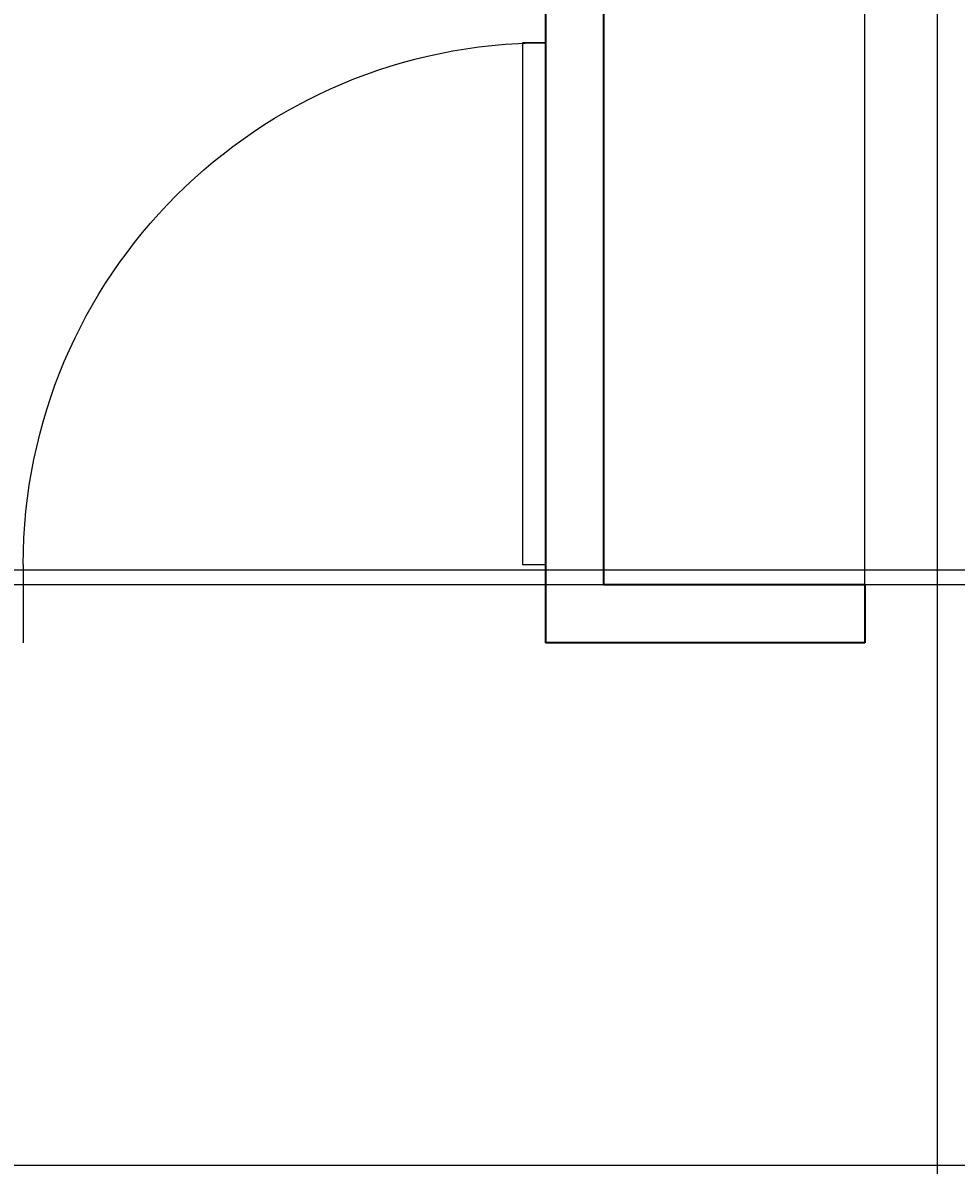
# Model space of a CAD drawing. Units: feet. Extents: x 105 to 1094, y -88 to 588.
# Tile 26 of 59: x 308 to 372, y 354 to 433. Entities that reach past the tile are written whole.
import ezdxf

# ---------------------------------------------------------------- set-up
doc = ezdxf.new("R2010")
doc.units = ezdxf.units.FT
doc.header["$MEASUREMENT"] = 0
for name, color, linetype, lineweight in [('A-ANNO-DIMS', 2, 'Continuous', 18), ('A-DOOR', 3, 'Continuous', 25), ('A-WALL', 7, 'Continuous', 35)]:
    doc.layers.add(name, color=color, linetype=linetype, lineweight=lineweight)
doc.styles.get("Standard").update_dxf_attribs({"font": 'arial.ttf'})
doc.dimstyles.get("Standard").update_dxf_attribs({"dimtxt": 0.18, "dimasz": 0.18, "dimexe": 0.18, "dimexo": 0.0625, "dimgap": 0.09, "dimtad": 0, "dimtih": 1, "dimtoh": 1, "dimdec": 4, "dimzin": 0, "dimdsep": 46, "dimtxsty": 'Standard', "dimcen": 0.09, "dimadec": 0, "dimazin": 0, "dimtfac": 1, "dimtdec": 4, "dimtofl": 0, "dimtmove": 0, "dimatfit": 3, "dimfxl": 1, "dimtolj": 1, "dimtzin": 0, "dimarcsym": 0})

# ---------------------------------------------------------------- blocks, each defined once
blk = doc.blocks.new('*U2')
for p, q in [((0, 0), (0, -6)), ((40, 0), (40, -6))]:
    blk.add_line(p, q)
blk.add_lwpolyline([(0, 0), (0, 40), (1.75, 40), (1.75, 0)], close=True)
blk.add_arc((0, 0), 40, 0, 90)
blk = doc.blocks.new('*D21')
at = {"layer": 'A-ANNO-DIMS', "color": 0, "lineweight": -2, "transparency": 16777216}
for p, q in [((849.626, 543.081), (105.458, 543.081)), ((105.638, 542.901), (105.638, 250.263)), ((105.638, -42.739), (105.638, 249.899)), ((849.626, -42.919), (105.458, -42.919))]:
    blk.add_line(p, q, dxfattribs=at)
at = {"layer": 'A-ANNO-DIMS', "color": 0, "transparency": 16777216}
for points in [[(105.608, 542.901), (105.668, 542.901), (105.638, 543.081)], [(105.608, -42.739), (105.668, -42.739), (105.638, -42.919)]]:
    blk.add_solid(points, dxfattribs=at)
at = {"layer": 'Defpoints', "color": 0, "transparency": 16777216}
for p in [(105.638, 543.081), (849.688, 543.081), (849.688, -42.919)]:
    blk.add_point(p, dxfattribs=at)
at = {"layer": 'A-ANNO-DIMS', "color": 0, "transparency": 16777216, "insert": (105.638, 250.081), "char_height": 0.18, "attachment_point": 5}
blk.add_mtext('\\A1;586', dxfattribs=at)
blk = doc.blocks.new('*D33')
at = {"layer": 'A-ANNO-DIMS', "color": 0, "lineweight": -2, "transparency": 16777216}
for p, q in [((646.626, 395.081), (105.458, 395.081)), ((105.638, 394.901), (105.638, 345.263)), ((105.638, 295.261), (105.638, 344.899)), ((646.626, 295.081), (105.458, 295.081))]:
    blk.add_line(p, q, dxfattribs=at)
at = {"layer": 'A-ANNO-DIMS', "color": 0, "transparency": 16777216}
for points in [[(105.608, 394.901), (105.668, 394.901), (105.638, 395.081)], [(105.608, 295.261), (105.668, 295.261), (105.638, 295.081)]]:
    blk.add_solid(points, dxfattribs=at)
at = {"layer": 'Defpoints', "color": 0, "transparency": 16777216}
for p in [(646.688, 395.081), (105.638, 295.081), (646.688, 295.081)]:
    blk.add_point(p, dxfattribs=at)
at = {"layer": 'A-ANNO-DIMS', "color": 0, "transparency": 16777216, "insert": (105.638, 345.081), "char_height": 0.18, "attachment_point": 5}
blk.add_mtext('\\A1;100', dxfattribs=at)
blk = doc.blocks.new('*D39')
at = {"layer": 'A-ANNO-DIMS', "color": 0, "lineweight": -2, "transparency": 16777216}
for p, q in [((294.688, 204.144), (294.688, 588.311)), ((294.868, 588.131), (332.47, 588.131)), ((370.508, 588.131), (332.906, 588.131)), ((370.688, 204.144), (370.688, 588.311))]:
    blk.add_line(p, q, dxfattribs=at)
at = {"layer": 'A-ANNO-DIMS', "color": 0, "transparency": 16777216}
for points in [[(294.868, 588.161), (294.868, 588.101), (294.688, 588.131)], [(370.508, 588.161), (370.508, 588.101), (370.688, 588.131)]]:
    blk.add_solid(points, dxfattribs=at)
at = {"layer": 'Defpoints', "color": 0, "transparency": 16777216}
for p in [(370.688, 588.131), (294.688, 204.081), (370.688, 204.081)]:
    blk.add_point(p, dxfattribs=at)
at = {"layer": 'A-ANNO-DIMS', "color": 0, "transparency": 16777216, "insert": (332.688, 588.131), "char_height": 0.18, "attachment_point": 5}
blk.add_mtext('\\A1;76', dxfattribs=at)
blk = doc.blocks.new('*D51')
at = {"layer": 'A-ANNO-DIMS', "color": 0, "lineweight": -2, "transparency": 16777216}
for p, q in [((432.626, 394.081), (105.458, 394.081)), ((105.638, 393.901), (105.638, 374.263)), ((105.638, 354.261), (105.638, 373.899)), ((426.626, 354.081), (105.458, 354.081))]:
    blk.add_line(p, q, dxfattribs=at)
at = {"layer": 'A-ANNO-DIMS', "color": 0, "transparency": 16777216}
for points in [[(105.608, 393.901), (105.668, 393.901), (105.638, 394.081)], [(105.608, 354.261), (105.668, 354.261), (105.638, 354.081)]]:
    blk.add_solid(points, dxfattribs=at)
at = {"layer": 'Defpoints', "color": 0, "transparency": 16777216}
for p in [(432.688, 394.081), (105.638, 354.081), (426.688, 354.081)]:
    blk.add_point(p, dxfattribs=at)
at = {"layer": 'A-ANNO-DIMS', "color": 0, "transparency": 16777216, "insert": (105.638, 374.081), "char_height": 0.18, "attachment_point": 5}
blk.add_mtext('\\A1;40', dxfattribs=at)
blk = doc.blocks.new('*D53')
at = {"layer": 'A-ANNO-DIMS', "color": 0, "lineweight": -2, "transparency": 16777216}
for p, q in [((365.688, 394.144), (365.688, 588.311)), ((365.868, 588.131), (389.966, 588.131)), ((414.508, 588.131), (390.411, 588.131)), ((414.688, 394.144), (414.688, 588.311))]:
    blk.add_line(p, q, dxfattribs=at)
at = {"layer": 'A-ANNO-DIMS', "color": 0, "transparency": 16777216}
for points in [[(365.868, 588.161), (365.868, 588.101), (365.688, 588.131)], [(414.508, 588.161), (414.508, 588.101), (414.688, 588.131)]]:
    blk.add_solid(points, dxfattribs=at)
at = {"layer": 'Defpoints', "color": 0, "transparency": 16777216}
for p in [(365.688, 588.131), (365.688, 394.081), (414.688, 394.081)]:
    blk.add_point(p, dxfattribs=at)
at = {"layer": 'A-ANNO-DIMS', "color": 0, "transparency": 16777216, "insert": (390.188, 588.131), "char_height": 0.18, "attachment_point": 5}
blk.add_mtext('\\A1;49', dxfattribs=at)

msp = doc.modelspace()

# ---------------------------------------------------------------- linework, layer by layer
at = {"layer": 'A-WALL'}
for p, q in [((343.6883, 507.0812), (343.6883, 390.0812)), ((347.6883, 491.0812), (347.6883, 394.0812)), ((365.6883, 394.0812), (347.6883, 394.0812)), ((365.6883, 394.0812), (365.6883, 390.0812)), ((365.6883, 390.0812), (343.6883, 390.0812))]:
    msp.add_line(p, q, dxfattribs=at)

# ---------------------------------------------------------------- block references
at = {"layer": 'A-DOOR', "xscale": -0.8984622266767051, "yscale": 0.8984622266767051, "zscale": 0.8984622266767051}
msp.add_blockref('*U2', (343.6883, 395.4719), dxfattribs=at)

# ---------------------------------------------------------------- dimensions: what is measured, and where the dimension line sits
at = {"layer": 'A-ANNO-DIMS'}
for base, p1, p2, picture, middle in [((370.6883, 588.1312), (294.6883, 204.0812), (370.6883, 204.0812), '*D39', (332.6883, 588.1312)), ((365.6883, 588.1312), (414.6883, 394.0812), (365.6883, 394.0812), '*D53', (390.1883, 588.1312))]:
    dim = msp.add_linear_dim(base=base, p1=p1, p2=p2, dimstyle='Standard', override={"dimdec": 0, "dimlfac": 1, "dimrnd": 0, "dimzin": 0, "dimdsep": 46, "dimlunit": 2}, dxfattribs=at)
    dim.commit()
    dim.dimension.update_dxf_attribs({"geometry": picture, "text_midpoint": middle})
for base, p1, p2, picture, middle in [((105.6383, 543.0812), (849.6883, -42.9188), (849.6883, 543.0812), '*D21', (105.6383, 250.0812)), ((105.6383, 295.0812), (646.6883, 395.0812), (646.6883, 295.0812), '*D33', (105.6383, 345.0812)), ((105.6383, 354.0812), (432.6883, 394.0812), (426.6883, 354.0812), '*D51', (105.6383, 374.0812))]:
    dim = msp.add_linear_dim(base=base, p1=p1, p2=p2, angle=90, dimstyle='Standard', override={"dimdec": 0, "dimlfac": 1, "dimrnd": 0, "dimzin": 0, "dimdsep": 46, "dimlunit": 2}, dxfattribs=at)
    dim.commit()
    dim.dimension.update_dxf_attribs({"geometry": picture, "text_midpoint": middle})

doc.saveas('drawing.dxf')
